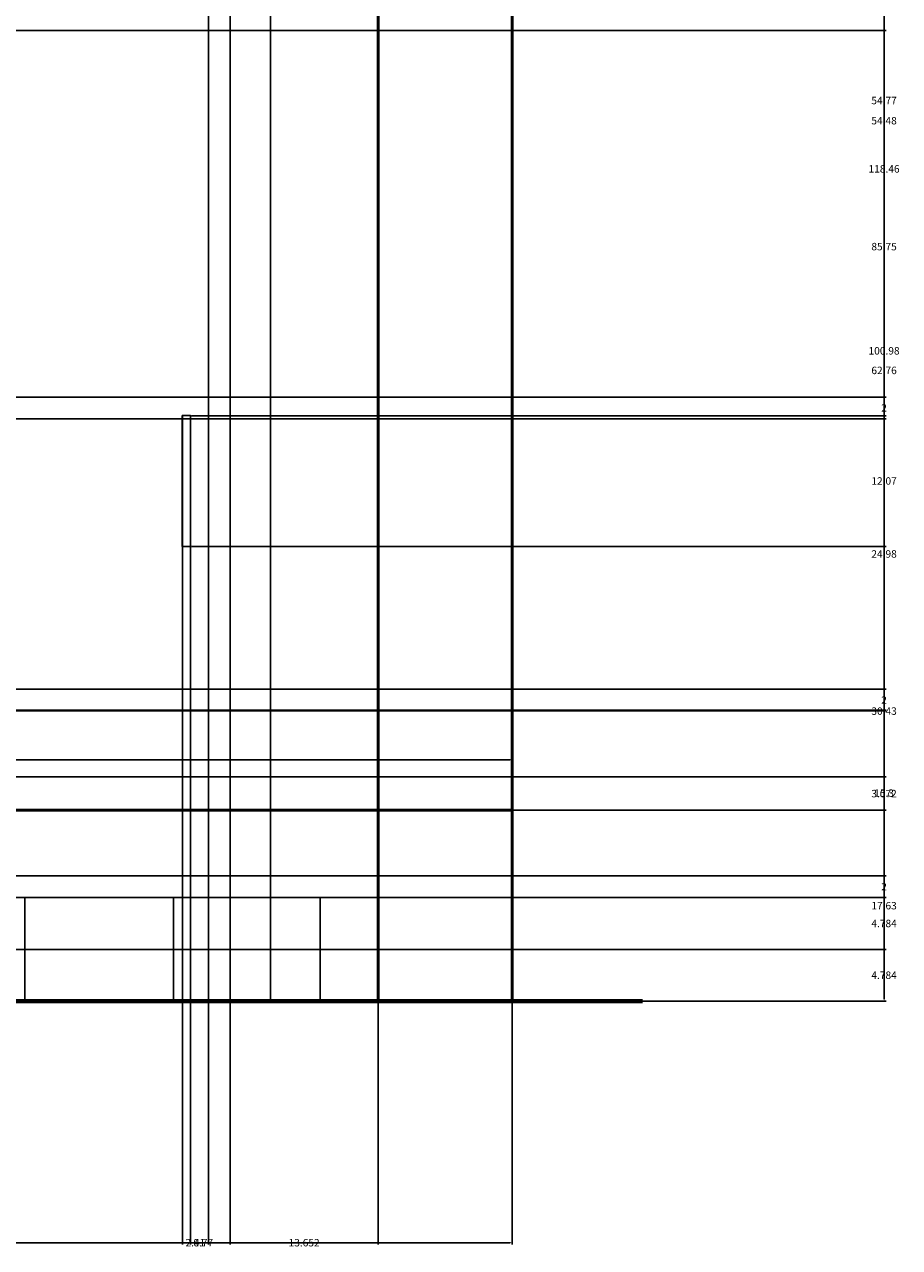
# Model space of a CAD drawing. Units: inches. Extents: x -139 to 346, y 72 to 413.
# Tile 13 of 18: x 265 to 346, y 72 to 185. Entities that reach past the tile are written whole.
import ezdxf

# ---------------------------------------------------------------- set-up
doc = ezdxf.new("R2010")
doc.units = ezdxf.units.IN
doc.header["$MEASUREMENT"] = 0
for name, color, linetype, lineweight in [('A-ANNO-DIMS', 2, 'Continuous', 18), ('A-DOOR', 3, 'Continuous', 25), ('A-FLOR-STRS', 2, 'Continuous', 25), ('A-WALL', 7, 'Continuous', 50), ('C-TOPO', 7, 'Continuous', 70)]:
    doc.layers.add(name, color=color, linetype=linetype, lineweight=lineweight)
doc.styles.get("Standard").update_dxf_attribs({"font": 'arial.ttf'})
doc.dimstyles.get("Standard").update_dxf_attribs({"dimtxt": 0.6875, "dimasz": 0.18, "dimexe": 0.18, "dimexo": 0.0625, "dimgap": 0.09, "dimtad": 0, "dimtih": 1, "dimtoh": 1, "dimdec": 4, "dimzin": 0, "dimdsep": 46, "dimlunit": 4, "dimtxsty": 'Standard', "dimcen": 0.09, "dimadec": 0, "dimazin": 0, "dimtfac": 1, "dimtdec": 4, "dimtofl": 0, "dimtmove": 0, "dimatfit": 3, "dimfxl": 1, "dimtolj": 1, "dimtzin": 0, "dimarcsym": 0})

# ---------------------------------------------------------------- blocks, each defined once
blk = doc.blocks.new('*D7')
at = {"layer": 'A-ANNO-DIMS', "color": 0, "lineweight": -2, "transparency": 16777216}
for p, q in [((-47.27, 95.04), (-47.27, 117.45)), ((-47.09, 117.27), (129.79, 117.27)), ((309.71, 117.27), (132.82, 117.27)), ((309.89, 95.04), (309.89, 117.45))]:
    blk.add_line(p, q, dxfattribs=at)
at = {"layer": 'A-ANNO-DIMS', "color": 0, "transparency": 16777216}
for points in [[(-47.09, 117.3), (-47.09, 117.24), (-47.27, 117.27)], [(309.71, 117.3), (309.71, 117.24), (309.89, 117.27)]]:
    blk.add_solid(points, dxfattribs=at)
at = {"layer": 'Defpoints', "color": 0, "transparency": 16777216}
for p in [(309.89, 117.27), (-47.27, 94.97), (309.89, 94.97)]:
    blk.add_point(p, dxfattribs=at)
at = {"layer": 'A-ANNO-DIMS', "color": 0, "transparency": 16777216, "insert": (131.31, 117.27), "char_height": 0.688, "attachment_point": 5}
blk.add_mtext('\\A1;357.16', dxfattribs=at)
blk = doc.blocks.new('*D11')
at = {"layer": 'A-ANNO-DIMS', "color": 0, "lineweight": -2, "transparency": 16777216}
for p, q in [((112.65, 112.54), (112.65, 72.49)), ((309.89, 94.91), (309.89, 72.49)), ((112.83, 72.67), (209.79, 72.67)), ((309.71, 72.67), (212.75, 72.67))]:
    blk.add_line(p, q, dxfattribs=at)
at = {"layer": 'A-ANNO-DIMS', "color": 0, "transparency": 16777216}
for points in [[(112.83, 72.7), (112.83, 72.64), (112.65, 72.67)], [(309.71, 72.7), (309.71, 72.64), (309.89, 72.67)]]:
    blk.add_solid(points, dxfattribs=at)
at = {"layer": 'Defpoints', "color": 0, "transparency": 16777216}
for p in [(112.65, 112.6), (309.89, 94.97), (309.89, 72.67)]:
    blk.add_point(p, dxfattribs=at)
at = {"layer": 'A-ANNO-DIMS', "color": 0, "transparency": 16777216, "insert": (211.27, 72.67), "char_height": 0.688, "attachment_point": 5}
blk.add_mtext('\\A1;197.24', dxfattribs=at)
blk = doc.blocks.new('*D16')
at = {"layer": 'A-ANNO-DIMS', "color": 0, "lineweight": -2, "transparency": 16777216}
for p, q in [((125.31, 115.68), (344.39, 115.68)), ((344.21, 115.5), (344.21, 114.58)), ((344.21, 112.78), (344.21, 113.7)), ((112.71, 112.6), (344.39, 112.6))]:
    blk.add_line(p, q, dxfattribs=at)
at = {"layer": 'A-ANNO-DIMS', "color": 0, "transparency": 16777216}
for points in [[(344.18, 115.5), (344.24, 115.5), (344.21, 115.68)], [(344.18, 112.78), (344.24, 112.78), (344.21, 112.6)]]:
    blk.add_solid(points, dxfattribs=at)
at = {"layer": 'Defpoints', "color": 0, "transparency": 16777216}
for p in [(125.25, 115.68), (344.21, 115.68), (112.65, 112.6)]:
    blk.add_point(p, dxfattribs=at)
at = {"layer": 'A-ANNO-DIMS', "color": 0, "transparency": 16777216, "insert": (344.21, 114.14), "char_height": 0.688, "attachment_point": 5}
blk.add_mtext('\\A1;3.072', dxfattribs=at)
blk = doc.blocks.new('*D21')
at = {"layer": 'A-ANNO-DIMS', "color": 0, "lineweight": -2, "transparency": 16777216}
for p, q in [((229.97, 104.48), (229.97, 72.49)), ((283.85, 104.48), (283.85, 72.49)), ((230.15, 72.67), (255.66, 72.67)), ((283.67, 72.67), (258.16, 72.67))]:
    blk.add_line(p, q, dxfattribs=at)
at = {"layer": 'A-ANNO-DIMS', "color": 0, "transparency": 16777216}
for points in [[(230.15, 72.7), (230.15, 72.64), (229.97, 72.67)], [(283.67, 72.7), (283.67, 72.64), (283.85, 72.67)]]:
    blk.add_solid(points, dxfattribs=at)
at = {"layer": 'Defpoints', "color": 0, "transparency": 16777216}
for p in [(229.97, 104.54), (283.85, 104.54), (283.85, 72.67)]:
    blk.add_point(p, dxfattribs=at)
at = {"layer": 'A-ANNO-DIMS', "color": 0, "transparency": 16777216, "insert": (256.91, 72.67), "char_height": 0.688, "attachment_point": 5}
blk.add_mtext('\\A1;53.88', dxfattribs=at)
blk = doc.blocks.new('*D22')
at = {"layer": 'A-ANNO-DIMS', "color": 0, "lineweight": -2, "transparency": 16777216}
for p, q in [((283.85, 104.48), (283.85, 72.49)), ((297.5, 94.91), (297.5, 72.49)), ((284.03, 72.67), (289.19, 72.67)), ((297.32, 72.67), (292.16, 72.67))]:
    blk.add_line(p, q, dxfattribs=at)
at = {"layer": 'A-ANNO-DIMS', "color": 0, "transparency": 16777216}
for points in [[(284.03, 72.7), (284.03, 72.64), (283.85, 72.67)], [(297.32, 72.7), (297.32, 72.64), (297.5, 72.67)]]:
    blk.add_solid(points, dxfattribs=at)
at = {"layer": 'Defpoints', "color": 0, "transparency": 16777216}
for p in [(283.85, 104.54), (297.5, 94.97), (297.5, 72.67)]:
    blk.add_point(p, dxfattribs=at)
at = {"layer": 'A-ANNO-DIMS', "color": 0, "transparency": 16777216, "insert": (290.68, 72.67), "char_height": 0.688, "attachment_point": 5}
blk.add_mtext('\\A1;13.652', dxfattribs=at)
blk = doc.blocks.new('*D31')
at = {"layer": 'A-ANNO-DIMS', "color": 0, "lineweight": -2, "transparency": 16777216}
for p, q in [((309.83, 389.97), (287.41, 389.97)), ((287.59, 389.79), (287.59, 242.92)), ((287.59, 95.15), (287.59, 242.03)), ((309.83, 94.97), (287.41, 94.97))]:
    blk.add_line(p, q, dxfattribs=at)
at = {"layer": 'A-ANNO-DIMS', "color": 0, "transparency": 16777216}
for points in [[(287.56, 389.79), (287.62, 389.79), (287.59, 389.97)], [(287.56, 95.15), (287.62, 95.15), (287.59, 94.97)]]:
    blk.add_solid(points, dxfattribs=at)
at = {"layer": 'Defpoints', "color": 0, "transparency": 16777216}
for p in [(287.59, 389.97), (309.89, 389.97), (309.89, 94.97)]:
    blk.add_point(p, dxfattribs=at)
at = {"layer": 'A-ANNO-DIMS', "color": 0, "transparency": 16777216, "insert": (287.59, 242.47), "char_height": 0.688, "attachment_point": 5}
blk.add_mtext('\\A1;295', dxfattribs=at)
blk = doc.blocks.new('*D32')
at = {"layer": 'A-ANNO-DIMS', "color": 0, "lineweight": -2, "transparency": 16777216}
for p, q in [((309.95, 112.6), (344.39, 112.6)), ((344.21, 112.42), (344.21, 104.23)), ((344.21, 95.15), (344.21, 103.35)), ((309.95, 94.97), (344.39, 94.97))]:
    blk.add_line(p, q, dxfattribs=at)
at = {"layer": 'A-ANNO-DIMS', "color": 0, "transparency": 16777216}
for points in [[(344.18, 112.42), (344.24, 112.42), (344.21, 112.6)], [(344.18, 95.15), (344.24, 95.15), (344.21, 94.97)]]:
    blk.add_solid(points, dxfattribs=at)
at = {"layer": 'Defpoints', "color": 0, "transparency": 16777216}
for p in [(309.89, 112.6), (344.21, 112.6), (309.89, 94.97)]:
    blk.add_point(p, dxfattribs=at)
at = {"layer": 'A-ANNO-DIMS', "color": 0, "transparency": 16777216, "insert": (344.21, 103.79), "char_height": 0.688, "attachment_point": 5}
blk.add_mtext('\\A1;17.63', dxfattribs=at)
blk = doc.blocks.new('*D33')
at = {"layer": 'A-ANNO-DIMS', "color": 0, "lineweight": -2, "transparency": 16777216}
for p, q in [((297.56, 231.06), (344.39, 231.06)), ((344.21, 230.88), (344.21, 172.27)), ((344.21, 112.78), (344.21, 171.39)), ((309.95, 112.6), (344.39, 112.6))]:
    blk.add_line(p, q, dxfattribs=at)
at = {"layer": 'A-ANNO-DIMS', "color": 0, "transparency": 16777216}
for points in [[(344.18, 230.88), (344.24, 230.88), (344.21, 231.06)], [(344.18, 112.78), (344.24, 112.78), (344.21, 112.6)]]:
    blk.add_solid(points, dxfattribs=at)
at = {"layer": 'Defpoints', "color": 0, "transparency": 16777216}
for p in [(297.5, 231.06), (344.21, 231.06), (309.89, 112.6)]:
    blk.add_point(p, dxfattribs=at)
at = {"layer": 'A-ANNO-DIMS', "color": 0, "transparency": 16777216, "insert": (344.21, 171.83), "char_height": 0.688, "attachment_point": 5}
blk.add_mtext('\\A1;118.46', dxfattribs=at)
blk = doc.blocks.new('*D62')
at = {"layer": 'A-ANNO-DIMS', "color": 0, "lineweight": -2, "transparency": 16777216}
for p, q in [((55.33, 123.78), (344.39, 123.78)), ((344.21, 123.6), (344.21, 123.21)), ((344.21, 121.96), (344.21, 122.34)), ((57.33, 121.78), (344.39, 121.78))]:
    blk.add_line(p, q, dxfattribs=at)
at = {"layer": 'A-ANNO-DIMS', "color": 0, "transparency": 16777216}
for points in [[(344.18, 123.6), (344.24, 123.6), (344.21, 123.78)], [(344.18, 121.96), (344.24, 121.96), (344.21, 121.78)]]:
    blk.add_solid(points, dxfattribs=at)
at = {"layer": 'Defpoints', "color": 0, "transparency": 16777216}
for p in [(55.27, 123.78), (344.21, 123.78), (57.27, 121.78)]:
    blk.add_point(p, dxfattribs=at)
at = {"layer": 'A-ANNO-DIMS', "color": 0, "transparency": 16777216, "insert": (344.21, 122.78), "char_height": 0.688, "attachment_point": 5}
blk.add_mtext('\\A1;2', dxfattribs=at)
blk = doc.blocks.new('*D63')
at = {"layer": 'A-ANNO-DIMS', "color": 0, "lineweight": -2, "transparency": 16777216}
for p, q in [((55.33, 148.76), (344.39, 148.76)), ((344.21, 148.58), (344.21, 136.71)), ((344.21, 123.96), (344.21, 135.83)), ((55.33, 123.78), (344.39, 123.78))]:
    blk.add_line(p, q, dxfattribs=at)
at = {"layer": 'A-ANNO-DIMS', "color": 0, "transparency": 16777216}
for points in [[(344.18, 148.58), (344.24, 148.58), (344.21, 148.76)], [(344.18, 123.96), (344.24, 123.96), (344.21, 123.78)]]:
    blk.add_solid(points, dxfattribs=at)
at = {"layer": 'Defpoints', "color": 0, "transparency": 16777216}
for p in [(55.27, 148.76), (344.21, 148.76), (55.27, 123.78)]:
    blk.add_point(p, dxfattribs=at)
at = {"layer": 'A-ANNO-DIMS', "color": 0, "transparency": 16777216, "insert": (344.21, 136.27), "char_height": 0.688, "attachment_point": 5}
blk.add_mtext('\\A1;24.98', dxfattribs=at)
blk = doc.blocks.new('*D64')
at = {"layer": 'A-ANNO-DIMS', "color": 0, "lineweight": -2, "transparency": 16777216}
for p, q in [((55.33, 150.76), (344.39, 150.76)), ((344.21, 150.58), (344.21, 150.19)), ((344.21, 148.94), (344.21, 149.32)), ((55.33, 148.76), (344.39, 148.76))]:
    blk.add_line(p, q, dxfattribs=at)
at = {"layer": 'A-ANNO-DIMS', "color": 0, "transparency": 16777216}
for points in [[(344.18, 150.58), (344.24, 150.58), (344.21, 150.76)], [(344.18, 148.94), (344.24, 148.94), (344.21, 148.76)]]:
    blk.add_solid(points, dxfattribs=at)
at = {"layer": 'Defpoints', "color": 0, "transparency": 16777216}
for p in [(55.27, 150.76), (344.21, 150.76), (55.27, 148.76)]:
    blk.add_point(p, dxfattribs=at)
at = {"layer": 'A-ANNO-DIMS', "color": 0, "transparency": 16777216, "insert": (344.21, 149.76), "char_height": 0.688, "attachment_point": 5}
blk.add_mtext('\\A1;2', dxfattribs=at)
blk = doc.blocks.new('*D65')
at = {"layer": 'A-ANNO-DIMS', "color": 0, "lineweight": -2, "transparency": 16777216}
for p, q in [((55.33, 205.52), (344.39, 205.52)), ((344.21, 205.34), (344.21, 178.58)), ((344.21, 150.94), (344.21, 177.7)), ((55.33, 150.76), (344.39, 150.76))]:
    blk.add_line(p, q, dxfattribs=at)
at = {"layer": 'A-ANNO-DIMS', "color": 0, "transparency": 16777216}
for points in [[(344.18, 205.34), (344.24, 205.34), (344.21, 205.52)], [(344.18, 150.94), (344.24, 150.94), (344.21, 150.76)]]:
    blk.add_solid(points, dxfattribs=at)
at = {"layer": 'Defpoints', "color": 0, "transparency": 16777216}
for p in [(55.27, 205.52), (344.21, 205.52), (55.27, 150.76)]:
    blk.add_point(p, dxfattribs=at)
at = {"layer": 'A-ANNO-DIMS', "color": 0, "transparency": 16777216, "insert": (344.21, 178.14), "char_height": 0.688, "attachment_point": 5}
blk.add_mtext('\\A1;54.77', dxfattribs=at)
blk = doc.blocks.new('*D67')
at = {"layer": 'A-ANNO-DIMS', "color": 0, "lineweight": -2, "transparency": 16777216}
for p, q in [((57.33, 207.52), (344.39, 207.52)), ((344.21, 207.34), (344.21, 165.09)), ((344.21, 121.96), (344.21, 164.21)), ((57.33, 121.78), (344.39, 121.78))]:
    blk.add_line(p, q, dxfattribs=at)
at = {"layer": 'A-ANNO-DIMS', "color": 0, "transparency": 16777216}
for points in [[(344.18, 207.34), (344.24, 207.34), (344.21, 207.52)], [(344.18, 121.96), (344.24, 121.96), (344.21, 121.78)]]:
    blk.add_solid(points, dxfattribs=at)
at = {"layer": 'Defpoints', "color": 0, "transparency": 16777216}
for p in [(57.27, 207.52), (344.21, 207.52), (57.27, 121.78)]:
    blk.add_point(p, dxfattribs=at)
at = {"layer": 'A-ANNO-DIMS', "color": 0, "transparency": 16777216, "insert": (344.21, 164.65), "char_height": 0.688, "attachment_point": 5}
blk.add_mtext('\\A1;85.75', dxfattribs=at)
blk = doc.blocks.new('*D74')
at = {"layer": 'A-ANNO-DIMS', "color": 0, "lineweight": -2, "transparency": 16777216}
for p, q in [((283.91, 205.52), (344.39, 205.52)), ((344.21, 205.34), (344.21, 155.47)), ((344.21, 104.72), (344.21, 154.59)), ((283.91, 104.54), (344.39, 104.54))]:
    blk.add_line(p, q, dxfattribs=at)
at = {"layer": 'A-ANNO-DIMS', "color": 0, "transparency": 16777216}
for points in [[(344.18, 205.34), (344.24, 205.34), (344.21, 205.52)], [(344.18, 104.72), (344.24, 104.72), (344.21, 104.54)]]:
    blk.add_solid(points, dxfattribs=at)
at = {"layer": 'Defpoints', "color": 0, "transparency": 16777216}
for p in [(283.85, 205.52), (344.21, 205.52), (283.85, 104.54)]:
    blk.add_point(p, dxfattribs=at)
at = {"layer": 'A-ANNO-DIMS', "color": 0, "transparency": 16777216, "insert": (344.21, 155.03), "char_height": 0.688, "attachment_point": 5}
blk.add_mtext('\\A1;100.98', dxfattribs=at)
blk = doc.blocks.new('*D75')
at = {"layer": 'A-ANNO-DIMS', "color": 0, "lineweight": -2, "transparency": 16777216}
for p, q in [((281.91, 106.54), (344.39, 106.54)), ((344.21, 106.36), (344.21, 105.98)), ((344.21, 104.72), (344.21, 105.11)), ((283.91, 104.54), (344.39, 104.54))]:
    blk.add_line(p, q, dxfattribs=at)
at = {"layer": 'A-ANNO-DIMS', "color": 0, "transparency": 16777216}
for points in [[(344.18, 106.36), (344.24, 106.36), (344.21, 106.54)], [(344.18, 104.72), (344.24, 104.72), (344.21, 104.54)]]:
    blk.add_solid(points, dxfattribs=at)
at = {"layer": 'Defpoints', "color": 0, "transparency": 16777216}
for p in [(281.85, 106.54), (344.21, 106.54), (283.85, 104.54)]:
    blk.add_point(p, dxfattribs=at)
at = {"layer": 'A-ANNO-DIMS', "color": 0, "transparency": 16777216, "insert": (344.21, 105.54), "char_height": 0.688, "attachment_point": 5}
blk.add_mtext('\\A1;2', dxfattribs=at)
blk = doc.blocks.new('*D76')
at = {"layer": 'A-ANNO-DIMS', "color": 0, "lineweight": -2, "transparency": 16777216}
for p, q in [((280.27, 136.97), (344.39, 136.97)), ((344.21, 136.79), (344.21, 122.2)), ((344.21, 106.72), (344.21, 121.32)), ((281.91, 106.54), (344.39, 106.54))]:
    blk.add_line(p, q, dxfattribs=at)
at = {"layer": 'A-ANNO-DIMS', "color": 0, "transparency": 16777216}
for points in [[(344.18, 136.79), (344.24, 136.79), (344.21, 136.97)], [(344.18, 106.72), (344.24, 106.72), (344.21, 106.54)]]:
    blk.add_solid(points, dxfattribs=at)
at = {"layer": 'Defpoints', "color": 0, "transparency": 16777216}
for p in [(280.2, 136.97), (344.21, 136.97), (281.85, 106.54)]:
    blk.add_point(p, dxfattribs=at)
at = {"layer": 'A-ANNO-DIMS', "color": 0, "transparency": 16777216, "insert": (344.21, 121.76), "char_height": 0.688, "attachment_point": 5}
blk.add_mtext('\\A1;30.43', dxfattribs=at)
blk = doc.blocks.new('*D77')
at = {"layer": 'A-ANNO-DIMS', "color": 0, "lineweight": -2, "transparency": 16777216}
for p, q in [((280.27, 149.04), (344.39, 149.04)), ((344.21, 148.86), (344.21, 143.45)), ((344.21, 137.15), (344.21, 142.57)), ((280.27, 136.97), (344.39, 136.97))]:
    blk.add_line(p, q, dxfattribs=at)
at = {"layer": 'A-ANNO-DIMS', "color": 0, "transparency": 16777216}
for points in [[(344.18, 148.86), (344.24, 148.86), (344.21, 149.04)], [(344.18, 137.15), (344.24, 137.15), (344.21, 136.97)]]:
    blk.add_solid(points, dxfattribs=at)
at = {"layer": 'Defpoints', "color": 0, "transparency": 16777216}
for p in [(280.2, 149.04), (344.21, 149.04), (280.2, 136.97)]:
    blk.add_point(p, dxfattribs=at)
at = {"layer": 'A-ANNO-DIMS', "color": 0, "transparency": 16777216, "insert": (344.21, 143.01), "char_height": 0.688, "attachment_point": 5}
blk.add_mtext('\\A1;12.07', dxfattribs=at)
blk = doc.blocks.new('*D78')
at = {"layer": 'A-ANNO-DIMS', "color": 0, "lineweight": -2, "transparency": 16777216}
for p, q in [((281.91, 203.52), (344.39, 203.52)), ((344.21, 203.34), (344.21, 176.72)), ((344.21, 149.22), (344.21, 175.84)), ((280.27, 149.04), (344.39, 149.04))]:
    blk.add_line(p, q, dxfattribs=at)
at = {"layer": 'A-ANNO-DIMS', "color": 0, "transparency": 16777216}
for points in [[(344.18, 203.34), (344.24, 203.34), (344.21, 203.52)], [(344.18, 149.22), (344.24, 149.22), (344.21, 149.04)]]:
    blk.add_solid(points, dxfattribs=at)
at = {"layer": 'Defpoints', "color": 0, "transparency": 16777216}
for p in [(281.85, 203.52), (344.21, 203.52), (280.2, 149.04)]:
    blk.add_point(p, dxfattribs=at)
at = {"layer": 'A-ANNO-DIMS', "color": 0, "transparency": 16777216, "insert": (344.21, 176.28), "char_height": 0.688, "attachment_point": 5}
blk.add_mtext('\\A1;54.48', dxfattribs=at)
blk = doc.blocks.new('*D83')
at = {"layer": 'A-ANNO-DIMS', "color": 0, "lineweight": -2, "transparency": 16777216}
for p, q in [((245.9, 121.84), (344.39, 121.84)), ((344.21, 121.66), (344.21, 114.63)), ((344.21, 106.72), (344.21, 113.75)), ((232.03, 106.54), (344.39, 106.54))]:
    blk.add_line(p, q, dxfattribs=at)
at = {"layer": 'A-ANNO-DIMS', "color": 0, "transparency": 16777216}
for points in [[(344.18, 121.66), (344.24, 121.66), (344.21, 121.84)], [(344.18, 106.72), (344.24, 106.72), (344.21, 106.54)]]:
    blk.add_solid(points, dxfattribs=at)
at = {"layer": 'Defpoints', "color": 0, "transparency": 16777216}
for p in [(245.84, 121.84), (344.21, 121.84), (231.97, 106.54)]:
    blk.add_point(p, dxfattribs=at)
at = {"layer": 'A-ANNO-DIMS', "color": 0, "transparency": 16777216, "insert": (344.21, 114.19), "char_height": 0.688, "attachment_point": 5}
blk.add_mtext('\\A1;15.3', dxfattribs=at)
blk = doc.blocks.new('*D84')
at = {"layer": 'A-ANNO-DIMS', "color": 0, "lineweight": -2, "transparency": 16777216}
for p, q in [((245.9, 184.61), (344.39, 184.61)), ((344.21, 184.43), (344.21, 153.67)), ((344.21, 122.02), (344.21, 152.78)), ((245.9, 121.84), (344.39, 121.84))]:
    blk.add_line(p, q, dxfattribs=at)
at = {"layer": 'A-ANNO-DIMS', "color": 0, "transparency": 16777216}
for points in [[(344.18, 184.43), (344.24, 184.43), (344.21, 184.61)], [(344.18, 122.02), (344.24, 122.02), (344.21, 121.84)]]:
    blk.add_solid(points, dxfattribs=at)
at = {"layer": 'Defpoints', "color": 0, "transparency": 16777216}
for p in [(245.84, 184.61), (344.21, 184.61), (245.84, 121.84)]:
    blk.add_point(p, dxfattribs=at)
at = {"layer": 'A-ANNO-DIMS', "color": 0, "transparency": 16777216, "insert": (344.21, 153.22), "char_height": 0.688, "attachment_point": 5}
blk.add_mtext('\\A1;62.76', dxfattribs=at)
blk = doc.blocks.new('*D85')
at = {"layer": 'A-ANNO-DIMS', "color": 0, "lineweight": -2, "transparency": 16777216}
for p, q in [((279.44, 136.91), (279.44, 72.49)), ((280.2, 136.91), (280.2, 72.49)), ((279.62, 72.67), (280.02, 72.67)), ((280.2, 72.67), (280.38, 72.67))]:
    blk.add_line(p, q, dxfattribs=at)
at = {"layer": 'A-ANNO-DIMS', "color": 0, "transparency": 16777216}
for points in [[(279.62, 72.7), (279.62, 72.64), (279.44, 72.67)], [(280.02, 72.7), (280.02, 72.64), (280.2, 72.67)]]:
    blk.add_solid(points, dxfattribs=at)
at = {"layer": 'Defpoints', "color": 0, "transparency": 16777216}
for p in [(279.44, 136.97), (280.2, 136.97), (280.2, 72.67)]:
    blk.add_point(p, dxfattribs=at)
at = {"layer": 'A-ANNO-DIMS', "color": 0, "transparency": 16777216, "insert": (281.37, 72.67), "char_height": 0.688, "attachment_point": 5}
blk.add_mtext('\\A1;0.77', dxfattribs=at)
blk = doc.blocks.new('*D86')
at = {"layer": 'A-ANNO-DIMS', "color": 0, "lineweight": -2, "transparency": 16777216}
for p, q in [((281.85, 203.46), (281.85, 72.49)), ((279.44, 148.98), (279.44, 72.49)), ((279.62, 72.67), (279.72, 72.67)), ((281.67, 72.67), (281.57, 72.67))]:
    blk.add_line(p, q, dxfattribs=at)
at = {"layer": 'A-ANNO-DIMS', "color": 0, "transparency": 16777216}
for points in [[(279.62, 72.7), (279.62, 72.64), (279.44, 72.67)], [(281.67, 72.7), (281.67, 72.64), (281.85, 72.67)]]:
    blk.add_solid(points, dxfattribs=at)
at = {"layer": 'Defpoints', "color": 0, "transparency": 16777216}
for p in [(281.85, 203.52), (279.44, 149.04), (281.85, 72.67)]:
    blk.add_point(p, dxfattribs=at)
at = {"layer": 'A-ANNO-DIMS', "color": 0, "transparency": 16777216, "insert": (280.64, 72.67), "char_height": 0.688, "attachment_point": 5}
blk.add_mtext('\\A1;2.41', dxfattribs=at)
blk = doc.blocks.new('*D87')
at = {"layer": 'A-ANNO-DIMS', "color": 0, "lineweight": -2, "transparency": 16777216}
for p, q in [((297.56, 99.76), (344.39, 99.76)), ((344.21, 99.58), (344.21, 97.81)), ((344.21, 95.15), (344.21, 96.93)), ((297.56, 94.97), (344.39, 94.97))]:
    blk.add_line(p, q, dxfattribs=at)
at = {"layer": 'A-ANNO-DIMS', "color": 0, "transparency": 16777216}
for points in [[(344.18, 99.58), (344.24, 99.58), (344.21, 99.76)], [(344.18, 95.15), (344.24, 95.15), (344.21, 94.97)]]:
    blk.add_solid(points, dxfattribs=at)
at = {"layer": 'Defpoints', "color": 0, "transparency": 16777216}
for p in [(297.5, 99.76), (344.21, 99.76), (297.5, 94.97)]:
    blk.add_point(p, dxfattribs=at)
at = {"layer": 'A-ANNO-DIMS', "color": 0, "transparency": 16777216, "insert": (344.21, 97.37), "char_height": 0.688, "attachment_point": 5}
blk.add_mtext('\\A1;4.784', dxfattribs=at)
blk = doc.blocks.new('*D88')
at = {"layer": 'A-ANNO-DIMS', "color": 0, "lineweight": -2, "transparency": 16777216}
for p, q in [((297.56, 104.54), (344.39, 104.54)), ((344.21, 104.36), (344.21, 102.59)), ((344.21, 99.94), (344.21, 101.71)), ((297.56, 99.76), (344.39, 99.76))]:
    blk.add_line(p, q, dxfattribs=at)
at = {"layer": 'A-ANNO-DIMS', "color": 0, "transparency": 16777216}
for points in [[(344.18, 104.36), (344.24, 104.36), (344.21, 104.54)], [(344.18, 99.94), (344.24, 99.94), (344.21, 99.76)]]:
    blk.add_solid(points, dxfattribs=at)
at = {"layer": 'Defpoints', "color": 0, "transparency": 16777216}
for p in [(297.5, 104.54), (344.21, 104.54), (297.5, 99.76)]:
    blk.add_point(p, dxfattribs=at)
at = {"layer": 'A-ANNO-DIMS', "color": 0, "transparency": 16777216, "insert": (344.21, 102.15), "char_height": 0.688, "attachment_point": 5}
blk.add_mtext('\\A1;4.784', dxfattribs=at)

msp = doc.modelspace()

# ---------------------------------------------------------------- linework, layer by layer
at = {"layer": 'A-DOOR'}
for points in [[(229.972, 205.5243), (283.8497, 205.5243), (283.8497, 104.5429), (229.972, 104.5429)], [(231.972, 203.5243), (281.8497, 203.5243), (281.8497, 106.5429), (231.972, 106.5429)], [(279.438, 149.0409), (280.2036, 149.0409), (280.2036, 136.9714), (279.438, 136.9714)]]:
    msp.add_lwpolyline(points, close=True, dxfattribs=at)
at = {"layer": 'A-FLOR-STRS'}
for p, q in [((264.9138, 104.5429), (264.9138, 94.9748)), ((278.6177, 104.5429), (278.6177, 94.9748)), ((283.8497, 104.5429), (292.1669, 104.5429)), ((292.1669, 104.5429), (292.1669, 94.9748)), ((292.1669, 104.5429), (297.5013, 104.5429)), ((205.1121, 99.7588), (292.1669, 99.7588)), ((292.1669, 99.7588), (297.5013, 99.7588))]:
    msp.add_line(p, q, dxfattribs=at)
at = {"layer": 'A-WALL'}
for p, q in [((309.8894, 94.9748), (309.8894, 382.9748)), ((297.5013, 94.9748), (297.5013, 231.0607)), ((112.6506, 112.6042), (297.5013, 112.6042)), ((297.5013, 112.6042), (309.8894, 112.6042))]:
    msp.add_line(p, q, dxfattribs=at)
at = {"layer": 'C-TOPO'}
msp.add_line((51.0187, 94.9748), (321.9055, 94.9748), dxfattribs=at)

# ---------------------------------------------------------------- dimensions: what is measured, and where the dimension line sits
at = {"layer": 'A-ANNO-DIMS'}
for base, p1, p2, override, picture, middle in [((287.5894, 389.9748), (309.8894, 94.9748), (309.8894, 389.9748), {"dimdec": 0, "dimlfac": 1, "dimrnd": 0, "dimzin": 0, "dimdsep": 46, "dimlunit": 2}, '*D31', (287.5894, 242.4748)), ((344.2055, 231.0607), (309.8894, 112.6042), (297.5013, 231.0607), {"dimdec": 2, "dimlfac": 1, "dimrnd": 0, "dimzin": 0, "dimdsep": 46, "dimlunit": 2}, '*D33', (344.2055, 171.8325)), ((344.2055, 207.5243), (57.2654, 121.7753), (57.2654, 207.5243), {"dimdec": 2, "dimlfac": 1, "dimrnd": 0, "dimzin": 0, "dimdsep": 46, "dimlunit": 2}, '*D67', (344.2055, 164.6498)), ((344.2055, 205.5243), (55.2654, 150.7576), (55.2654, 205.5243), {"dimdec": 2, "dimlfac": 1, "dimrnd": 0, "dimzin": 0, "dimdsep": 46, "dimlunit": 2}, '*D65', (344.2055, 178.141)), ((344.2055, 205.5243), (283.8497, 104.5429), (283.8497, 205.5243), {"dimdec": 2, "dimlfac": 1, "dimrnd": 0, "dimzin": 0, "dimdsep": 46, "dimlunit": 2}, '*D74', (344.2055, 155.0336)), ((344.2055, 203.5243), (280.2036, 149.0409), (281.8497, 203.5243), {"dimdec": 2, "dimlfac": 1, "dimrnd": 0, "dimzin": 0, "dimdsep": 46, "dimlunit": 2}, '*D78', (344.2055, 176.2826)), ((344.2055, 184.6055), (245.8399, 121.8428), (245.8399, 184.6055), {"dimdec": 2, "dimlfac": 1, "dimrnd": 0, "dimzin": 0, "dimdsep": 46, "dimlunit": 2}, '*D84', (344.2055, 153.2242)), ((344.2055, 150.7576), (55.2654, 148.7576), (55.2654, 150.7576), {"dimdec": 0, "dimlfac": 1, "dimrnd": 0, "dimzin": 0, "dimdsep": 46, "dimlunit": 2}, '*D64', (344.2055, 149.7576)), ((344.2055, 148.7576), (55.2654, 123.7753), (55.2654, 148.7576), {"dimdec": 2, "dimlfac": 1, "dimrnd": 0, "dimzin": 0, "dimdsep": 46, "dimlunit": 2}, '*D63', (344.2055, 136.2665)), ((344.2055, 149.0409), (280.2036, 136.9714), (280.2036, 149.0409), {"dimdec": 2, "dimlfac": 1, "dimrnd": 0, "dimzin": 0, "dimdsep": 46, "dimlunit": 2}, '*D77', (344.2055, 143.0061)), ((344.2055, 136.9714), (281.8497, 106.5429), (280.2036, 136.9714), {"dimdec": 2, "dimlfac": 1, "dimrnd": 0, "dimzin": 0, "dimdsep": 46, "dimlunit": 2}, '*D76', (344.2055, 121.7571)), ((344.2055, 123.7753), (57.2654, 121.7753), (55.2654, 123.7753), {"dimdec": 0, "dimlfac": 1, "dimrnd": 0, "dimzin": 0, "dimdsep": 46, "dimlunit": 2}, '*D62', (344.2055, 122.7753)), ((344.2055, 121.8428), (231.972, 106.5429), (245.8399, 121.8428), {"dimdec": 1, "dimlfac": 1, "dimrnd": 0, "dimzin": 0, "dimdsep": 46, "dimlunit": 2}, '*D83', (344.2055, 114.1929)), ((344.2055, 115.6761), (112.6506, 112.6042), (125.2464, 115.6761), {"dimdec": 3, "dimlfac": 1, "dimrnd": 0, "dimzin": 0, "dimdsep": 46, "dimlunit": 2}, '*D16', (344.2055, 114.1402)), ((344.2055, 112.6042), (309.8894, 94.9748), (309.8894, 112.6042), {"dimdec": 2, "dimlfac": 1, "dimrnd": 0, "dimzin": 0, "dimdsep": 46, "dimlunit": 2}, '*D32', (344.2055, 103.7895)), ((344.2055, 106.5429), (283.8497, 104.5429), (281.8497, 106.5429), {"dimdec": 0, "dimlfac": 1, "dimrnd": 0, "dimzin": 0, "dimdsep": 46, "dimlunit": 2}, '*D75', (344.2055, 105.5429)), ((344.2055, 104.5429), (297.5013, 99.7588), (297.5013, 104.5429), {"dimdec": 3, "dimlfac": 1, "dimrnd": 0, "dimzin": 0, "dimdsep": 46, "dimlunit": 2}, '*D88', (344.2055, 102.1508)), ((344.2055, 99.7588), (297.5013, 94.9748), (297.5013, 99.7588), {"dimdec": 3, "dimlfac": 1, "dimrnd": 0, "dimzin": 0, "dimdsep": 46, "dimlunit": 2}, '*D87', (344.2055, 97.3668))]:
    dim = msp.add_linear_dim(base=base, p1=p1, p2=p2, angle=90, dimstyle='Standard', override=override, dxfattribs=at)
    dim.commit()
    dim.dimension.update_dxf_attribs({"geometry": picture, "text_midpoint": middle})
for base, p1, p2, override, picture, middle in [((281.8497, 72.6748), (279.438, 149.0409), (281.8497, 203.5243), {"dimdec": 2, "dimlfac": 1, "dimrnd": 0, "dimzin": 0, "dimdsep": 46, "dimlunit": 2}, '*D86', (280.6438, 72.6748)), ((280.2036, 72.6748), (279.438, 136.9714), (280.2036, 136.9714), {"dimdec": 2, "dimlfac": 1, "dimrnd": 0, "dimzin": 0, "dimdsep": 46, "dimlunit": 2}, '*D85', (281.3665, 72.6748)), ((309.8894, 117.2748), (-47.2734, 94.9748), (309.8894, 94.9748), {"dimdec": 2, "dimlfac": 1, "dimrnd": 0, "dimzin": 0, "dimdsep": 46, "dimlunit": 2}, '*D7', (131.308, 117.2748)), ((309.8894, 72.6748), (112.6506, 112.6042), (309.8894, 94.9748), {"dimdec": 2, "dimlfac": 1, "dimrnd": 0, "dimzin": 0, "dimdsep": 46, "dimlunit": 2}, '*D11', (211.27, 72.6748)), ((283.8497, 72.6748), (229.972, 104.5429), (283.8497, 104.5429), {"dimdec": 2, "dimlfac": 1, "dimrnd": 0, "dimzin": 0, "dimdsep": 46, "dimlunit": 2}, '*D21', (256.9109, 72.6748)), ((297.5013, 72.6748), (283.8497, 104.5429), (297.5013, 94.9748), {"dimdec": 3, "dimlfac": 1, "dimrnd": 0, "dimzin": 0, "dimdsep": 46, "dimlunit": 2}, '*D22', (290.6755, 72.6748))]:
    dim = msp.add_linear_dim(base=base, p1=p1, p2=p2, dimstyle='Standard', override=override, dxfattribs=at)
    dim.commit()
    dim.dimension.update_dxf_attribs({"geometry": picture, "text_midpoint": middle})

doc.saveas('drawing.dxf')
